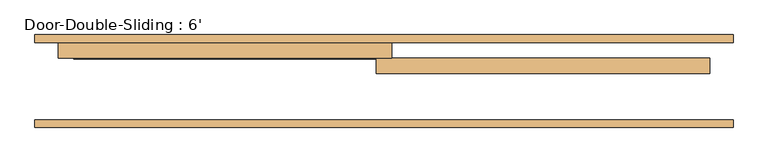
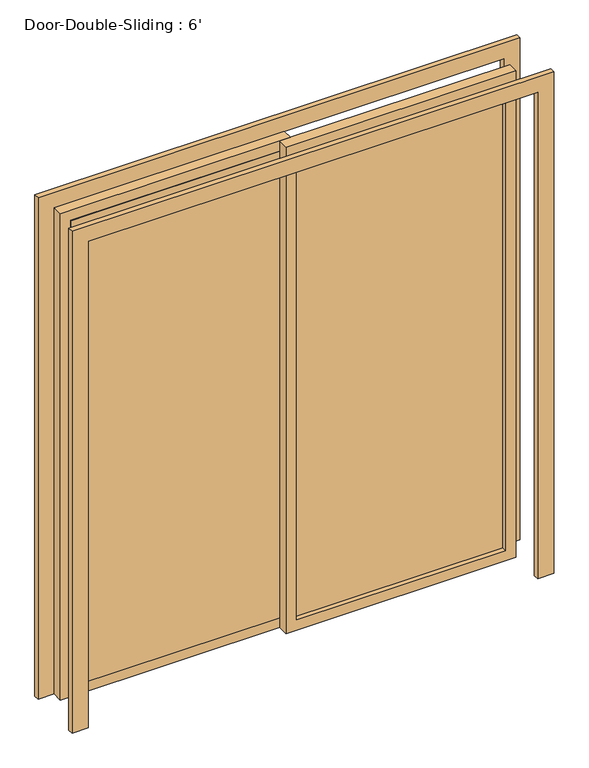
"""IFC4 building model written with IfcOpenShell, lengths in millimetres: door geometry, Door-Double-Sliding : 6'."""

from ifc_helpers import new_model, si_unit, frame, origin, place, context, project, spatial, polyline, outline, extrude, source, transform, mapped, element, save


def door_double_sliding_6_53f3f6b1(model_context):
    return source(origin(), model_context, "Body", "SweptSolid", [
        extrude(outline(polyline([(0.0, 1143.0), (2514.6, 1143.0), (2514.6, -1143.0), (0.0, -1143.0), (0.0, -1066.8), (2438.4, -1066.8), (2438.4, 1066.8), (0.0, 1066.8), (0.0, 1143.0)])), frame((0.0, 254.0, 0.0), z_axis=(0.0, 1.0, 0.0), x_axis=(0.0, 0.0, 1.0)), (0.0, 0.0, 1.0), 25.4),
        extrude(outline(polyline([(0.0, -1143.0), (0.0, -1066.8), (2438.4, -1066.8), (2438.4, 1066.8), (0.0, 1066.8), (0.0, 1143.0), (2514.6, 1143.0), (2514.6, -1143.0), (0.0, -1143.0)])), frame((0.0, -25.4, 0.0), z_axis=(0.0, 1.0, 0.0), x_axis=(0.0, 0.0, 1.0)), (0.0, 0.0, 1.0), 25.4),
        extrude(outline(polyline([(2438.4, 25.4), (2438.4, -1066.8), (0.0, -1066.8), (0.0, 25.4), (2438.4, 25.4)]), holes=[polyline([(2387.6, -25.4), (50.8, -25.4), (50.8, -1016.0), (2387.6, -1016.0), (2387.6, -25.4)])]), frame((0.0, 203.2, 0.0), z_axis=(0.0, 1.0, 0.0), x_axis=(0.0, 0.0, 1.0)), (0.0, 0.0, 1.0), 50.8),
        extrude(outline(polyline([(2438.4, -25.4), (0.0, -25.4), (0.0, 1066.8), (2438.4, 1066.8), (2438.4, -25.4)]), holes=[polyline([(2387.6, 25.4), (2387.6, 1016.0), (50.8, 1016.0), (50.8, 25.4), (2387.6, 25.4)])]), frame((0.0, 152.4, 0.0), z_axis=(0.0, 1.0, 0.0), x_axis=(0.0, 0.0, 1.0)), (0.0, 0.0, 1.0), 50.8),
        extrude(outline(polyline([(-25.4, 200.025), (-1016.0, 200.025), (-1016.0, 206.375), (-25.4, 206.375), (-25.4, 200.025)])), frame((0.0, 0.0, 50.8), z_axis=(0.0, 0.0, 1.0), x_axis=(1.0, 0.0, 0.0)), (0.0, 0.0, 1.0), 2336.8),
        extrude(outline(polyline([(25.4, 180.975), (1016.0, 180.975), (1016.0, 174.625), (25.4, 174.625), (25.4, 180.975)])), frame((0.0, 0.0, 50.8), z_axis=(0.0, 0.0, 1.0), x_axis=(1.0, 0.0, 0.0)), (0.0, 0.0, 1.0), 2336.8),
    ])


if __name__ == "__main__":
    model = new_model("IFC4")
    model_context = context("Model", 3, world=origin())
    ifc_project = project(units=[si_unit("LENGTHUNIT", "METRE", prefix="MILLI")], contexts=[model_context])
    site = spatial("IfcSite", under=ifc_project)
    building = spatial("IfcBuilding", under=site)
    placement = place(None, origin())
    door_double_sliding_6_shape = door_double_sliding_6_53f3f6b1(model_context)
    element("IfcDoor", 1, ObjectType="Door-Double-Sliding : 6'", at=placement, inside=building, context=model_context, shape_type="MappedRepresentation", body=[
        mapped(door_double_sliding_6_shape, transform((0.0, 0.0, 0.0), x_axis=(1.0, 0.0, 0.0), y_axis=(0.0, 1.0, 0.0), z_axis=(0.0, 0.0, 1.0))),
    ])
    save(model, "model.ifc")

# Revit data of these elements
# Type "Door-Double-Sliding : 6'"
#   Type Mark = "9"
#   Construction Type Id = "opn-d45"
#   Assembly Code = "C1020"
#   Analytic Construction = "Wood frame, double glass door "
#   Thickness = 0' - 2"
#   Thermal Resistance (R) = 1.8150 (h·ft²·°F)/BTU
#   Heat Transfer Coefficient (U) = 0.5510 BTU/(h·ft²·°F)
#   Height = 8' - 0"
#   Rail Width = 0' - 2"
#   Stiles = 0' - 2"
#   Trim Projection Ext = 0' - 1"
#   Trim Projection Int = 0' - 1"
#   Trim Width = 0' - 3"
#   Width = 7' - 0"
#   Define Thermal Properties by = 1
#   Glazing = Glass
#   Panel Material = Wood - Birch - Solid Stained Light Low Gloss
#   Trim Material = Paint - Sienna
#   Visual Light Transmittance = 0
#   Solar Heat Gain Coefficient = 0
#   Function = (empty or 0)
#   Wall Closure = (empty or 0)
# Element 1 (IfcDoor, "Door-Double-Sliding : 6'")
#   Materials on its faces: "Paint - Sienna", "Wood - Birch - Solid Stained Light Low Gloss", "Glass"
# Materials
#   "Glass": class "Glass", colour RGB 0 128 192, transparency 0.75, Description = "Soda Lime Glass", Cost = 0
#   "Wood - Birch - Solid Stained Light Low Gloss": class "Wood", colour RGB 210 159 95, transparency 0, Cost = 0
#   "Paint - Sienna": colour RGB 118 70 51, transparency 0, Cost = 0
